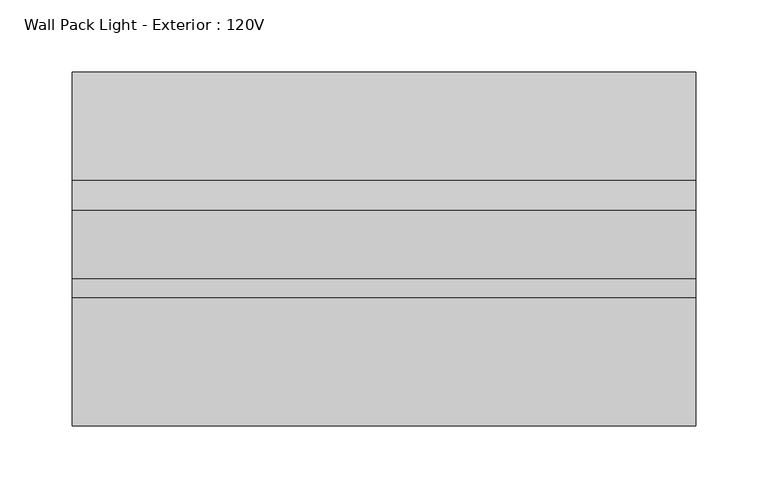
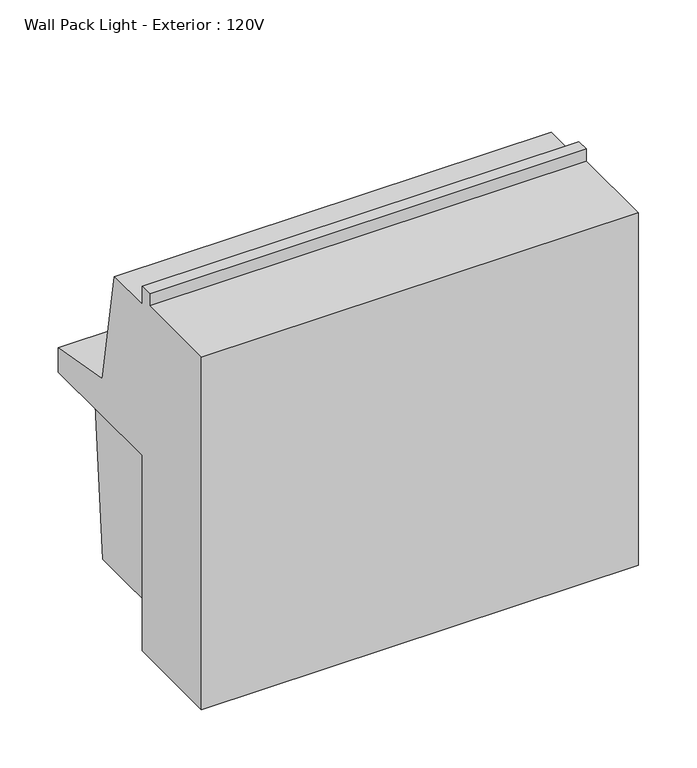
"""IFC4 building model written with IfcOpenShell, lengths in millimetres: light fixture geometry, Wall Pack Light - Exterior : 120V."""

from ifc_helpers import new_model, si_unit, frame, origin, place, context, project, spatial, polyline, outline, extrude, source, transform, mapped, element, save


def wall_pack_light_exterior_120v_663ef98a(model_context):
    return source(origin(), model_context, "Body", "SweptSolid", [
        extrude(outline(polyline([(190.5, 2755.9), (203.2, 2755.9), (203.2, 2736.85), (250.640971, 2736.85), (271.6426549, 2617.7435323), (346.6850056, 2604.5115412), (346.6850056, 2579.1115412), (203.2, 2579.1115412), (203.2, 2374.9), (101.6, 2374.9), (101.6, 2743.2), (190.5, 2743.2), (190.5, 2755.9)])), frame((-94.1359435, 0.0, 0.0), z_axis=(1.0, 0.0, 0.0), x_axis=(0.0, 1.0, 0.0)), (0.0, 0.0, 1.0), 431.8),
        extrude(outline(polyline([(315.020745, 2393.95), (203.2, 2393.95), (203.2, 2578.1), (330.1170754, 2578.1), (315.020745, 2393.95)])), frame((-68.7349223, 0.0, 0.0), z_axis=(1.0, 0.0, 0.0), x_axis=(0.0, 1.0, 0.0)), (0.0, 0.0, 1.0), 380.9989788),
    ])


if __name__ == "__main__":
    model = new_model("IFC4")
    model_context = context("Model", 3, world=origin())
    ifc_project = project(units=[si_unit("LENGTHUNIT", "METRE", prefix="MILLI")], contexts=[model_context])
    site = spatial("IfcSite", under=ifc_project)
    building = spatial("IfcBuilding", under=site)
    placement = place(None, origin())
    wall_pack_light_exterior_120v_shape = wall_pack_light_exterior_120v_663ef98a(model_context)
    element("IfcLightFixture", 1, ObjectType="Wall Pack Light - Exterior : 120V", at=placement, inside=building, context=model_context, shape_type="MappedRepresentation", body=[
        mapped(wall_pack_light_exterior_120v_shape, transform((0.0, 0.0, 0.0), x_axis=(1.0, 0.0, 0.0), y_axis=(0.0, 1.0, 0.0), z_axis=(0.0, 0.0, 1.0))),
    ])
    save(model, "model.ifc")

# Revit data of these elements
# Type "Wall Pack Light - Exterior : 120V"
#   Assembly Code = "D5020230"
#   Wattage = 300 W
#   built-in parameter 1150110 = 1 (stored number, unit not read)
#   built-in parameter 1114217 = 1 (stored number, unit not read)
#   built-in parameter 1150109 = 1 (stored number, unit not read)
#   built-in parameter 1150113 = 1 (stored number, unit not read)
#   built-in parameter 1150115 = 1 (stored number, unit not read)
#   built-in parameter 1150105 = 1875.72 (stored number, unit not read)
#   Light Source Symbol Size = 2' - 0"
#   built-in parameter 1150112 = 1 (stored number, unit not read)
#   built-in parameter 1150114 = 1 (stored number, unit not read)
#   built-in parameter 1150107 = 4000 (stored number, unit not read)
#   built-in parameter 1150106 = 18.7572 (stored number, unit not read)
#   built-in parameter 1150104 = 7.29939 (stored number, unit not read)
#   Ballast Voltage = 120 V
#   built-in parameter 1114218 = 1 (stored number, unit not read)
#   built-in parameter 1150133 = 10 (stored number, unit not read)
#   Lumens = 23571 lm
#   Mounting Height = 9' - 0"
#   Apparent Load = 70 VA
#   built-in parameter 1150134 = 12
#   built-in parameter 1150137 = 1
#   Color Filter = 16777215
#   Ballast Number of Poles = 1
#   Wall Mount Material = Metal - Paint Finish - Dark Grey, Matte
#   Shade Material = Glass
#   Load Classification = Lighting - Exterior
#   Dimming Lamp Color Temperature Shift = (empty or 0)
#   Default Elevation = 0
# Element 1 (IfcLightFixture, "Wall Pack Light - Exterior : 120V")
#   Materials on its faces: "Metal - Paint Finish - Dark Grey, Matte", "Glass"
# Materials
#   "Metal - Paint Finish - Dark Grey, Matte": class "Paint", colour RGB 98 98 98, transparency 0
#   "Glass": class "Glass", colour RGB 0 128 192, transparency 0.75, Description = "Soda Lime Glass", Cost = 0
